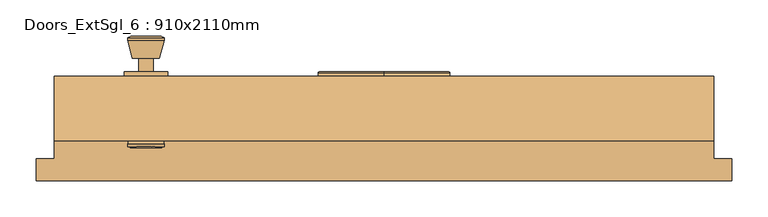
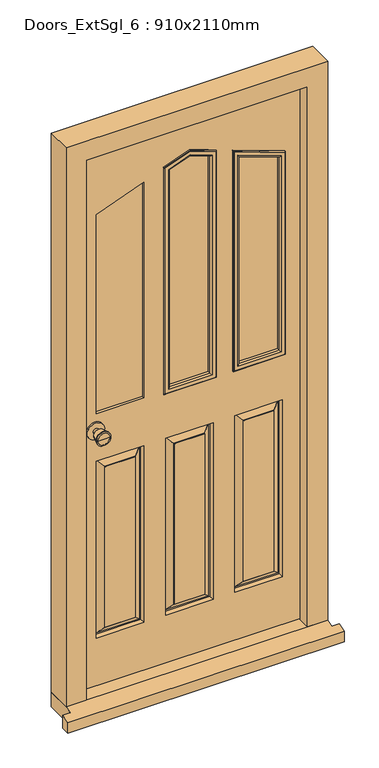
"""IFC4 building model written with IfcOpenShell, lengths in millimetres: door geometry, Doors_ExtSgl_6 : 910x2110mm."""

from ifc_helpers import new_model, si_unit, point, frame, frame_2d, origin, place, context, project, spatial, polyline, circle_curve, ellipse_curve, trimmed, segment, composite_curve, outline, extrude, faceted_brep, source, transform, mapped, element, save
from ifc_brep_helpers import plane_surface, cylinder_surface, revolved_surface, advanced_brep


def doors_extsgl_6_910x2110mm_72be2df1(model_context):
    return source(origin(), model_context, "Body", "SolidModel", [
        advanced_brep(
        [(-328.4666667, 18.4, 1000.0), (-338.4666667, 18.4, 1000.0), (-318.4666667, 18.4, 1000.0), (-307.9907991, 67.4, 1000.0), (-348.9425342, 67.4, 1000.0), (-328.4666667, 67.4, 1000.0), (-303.4666667, 65.5721319, 1000.0), (-353.4666667, 65.5721319, 1000.0), (-303.4666667, 62.1084537, 1000.0), (-353.4666667, 62.1084537, 1000.0), (-309.8304306, 37.4, 1000.0), (-347.1029027, 37.4, 1000.0), (-318.4666667, 37.4, 1000.0), (-338.4666667, 37.4, 1000.0)],
        [
            (0, 1),
            (1, 2, circle_curve(frame((-328.4666667, 18.4, 1000.0), z_axis=(0.0, -1.0, 0.0), x_axis=(-1.0, 0.0, 0.0)), 10.0)),
            (2, 0),
            (2, 1, circle_curve(frame((-328.4666667, 18.4, 1000.0), z_axis=(0.0, -1.0, 0.0), x_axis=(-1.0, 0.0, 0.0)), 10.0)),
            (3, 4, circle_curve(frame((-328.4666667, 67.4, 1000.0), z_axis=(0.0, 1.0, 0.0), x_axis=(-1.0, 0.0, 0.0)), 20.4758676)),
            (4, 5),
            (5, 3),
            (4, 3, circle_curve(frame((-328.4666667, 67.4, 1000.0), z_axis=(0.0, 1.0, 0.0), x_axis=(-1.0, 0.0, 0.0)), 20.4758676)),
            (6, 7, circle_curve(frame((-328.4666667, 65.5721319, 1000.0), z_axis=(0.0, 1.0, 0.0), x_axis=(-1.0, 0.0, 0.0)), 25.0)),
            (7, 4),
            (3, 6),
            (7, 6, circle_curve(frame((-328.4666667, 65.5721319, 1000.0), z_axis=(0.0, 1.0, 0.0), x_axis=(-1.0, 0.0, 0.0)), 25.0)),
            (8, 9, circle_curve(frame((-328.4666667, 62.1084537, 1000.0), z_axis=(0.0, 1.0, 0.0), x_axis=(-1.0, 0.0, 0.0)), 25.0)),
            (9, 7),
            (6, 8),
            (9, 8, circle_curve(frame((-328.4666667, 62.1084537, 1000.0), z_axis=(0.0, 1.0, 0.0), x_axis=(-1.0, 0.0, 0.0)), 25.0)),
            (10, 11, circle_curve(frame((-328.4666667, 37.4, 1000.0), z_axis=(0.0, 1.0, 0.0), x_axis=(-1.0, 0.0, 0.0)), 18.636236)),
            (11, 9),
            (8, 10),
            (11, 10, circle_curve(frame((-328.4666667, 37.4, 1000.0), z_axis=(0.0, 1.0, 0.0), x_axis=(-1.0, 0.0, 0.0)), 18.636236)),
            (12, 13, circle_curve(frame((-328.4666667, 37.4, 1000.0), z_axis=(0.0, 1.0, 0.0), x_axis=(-1.0, 0.0, 0.0)), 10.0)),
            (13, 11),
            (10, 12),
            (13, 12, circle_curve(frame((-328.4666667, 37.4, 1000.0), z_axis=(0.0, 1.0, 0.0), x_axis=(-1.0, 0.0, 0.0)), 10.0)),
            (1, 13),
            (12, 2),
        ],
        [
            plane_surface(frame((-328.4666667, 18.4, 1000.0), z_axis=(0.0, -1.0, 0.0), x_axis=(-1.0, 0.0, 0.0))),
            plane_surface(frame((-328.4666667, 67.4, 1000.0), z_axis=(0.0, 1.0, 0.0), x_axis=(-1.0, 0.0, 0.0))),
            revolved_surface(polyline([(-348.9425342, 67.4, 1000.0), (-353.4666667, 65.5721319, 1000.0)]), (-328.4666667, 18.4, 1000.0), (0.0, -1.0, 0.0)),
            cylinder_surface(frame((-328.4666667, 18.4, 1000.0), z_axis=(0.0, -1.0, 0.0), x_axis=(-1.0, 0.0, 0.0)), 25.0),
            revolved_surface(polyline([(-353.4666667, 62.1084537, 1000.0), (-347.1029027, 37.4, 1000.0)]), (-328.4666667, 18.4, 1000.0), (0.0, -1.0, 0.0)),
            plane_surface(frame((-328.4666667, 37.4, 1000.0), z_axis=(0.0, -1.0, 0.0), x_axis=(-1.0, 0.0, 0.0))),
            cylinder_surface(frame((-328.4666667, 18.4, 1000.0), z_axis=(0.0, -1.0, 0.0), x_axis=(-1.0, 0.0, 0.0)), 10.0),
        ],
        [
            (0, [[1, 2, 3]]),
            (0, [[-3, 4, -1]]),
            (1, [[5, 6, 7]]),
            (1, [[8, -7, -6]]),
            (2, [[9, 10, -5, 11]]),
            (2, [[12, -11, -8, -10]]),
            (3, [[13, 14, -9, 15]]),
            (3, [[16, -15, -12, -14]]),
            (4, [[17, 18, -13, 19]]),
            (4, [[20, -19, -16, -18]]),
            (5, [[21, 22, -17, 23]]),
            (5, [[24, -23, -20, -22]]),
            (6, [[-2, 25, -21, 26]]),
            (6, [[-4, -26, -24, -25]]),
        ],
    ),
        extrude(outline(composite_curve([segment(trimmed(circle_curve(frame_2d((1000.0, -328.4666667)), 30.0), [point((1000.0, -358.4666667))], [point((1000.0, -298.4666667))], False, "CARTESIAN"), True, "CONTINUOUS"), segment(trimmed(circle_curve(frame_2d((1000.0, -328.4666667)), 30.0), [point((1000.0, -298.4666667))], [point((1000.0, -358.4666667))], False, "CARTESIAN"), True, "CONTINUOUS")], self_intersect=False)), frame((0.0, 12.4, 0.0), z_axis=(0.0, 1.0, 0.0), x_axis=(0.0, 0.0, 1.0)), (0.0, 0.0, 1.0), 6.0),
        advanced_brep(
        [(-328.4666667, -37.6, 1000.0), (-318.4666667, -37.6, 1000.0), (-338.4666667, -37.6, 1000.0), (-307.9907991, -86.6, 1000.0), (-328.4666667, -86.6, 1000.0), (-348.9425342, -86.6, 1000.0), (-303.4666667, -84.7721319, 1000.0), (-353.4666667, -84.7721319, 1000.0), (-303.4666667, -81.3084537, 1000.0), (-353.4666667, -81.3084537, 1000.0), (-309.8304306, -56.6, 1000.0), (-347.1029027, -56.6, 1000.0), (-318.4666667, -56.6, 1000.0), (-338.4666667, -56.6, 1000.0)],
        [
            (0, 1),
            (1, 2, circle_curve(frame((-328.4666667, -37.6, 1000.0), z_axis=(0.0, 1.0, 0.0), x_axis=(-1.0, 0.0, 0.0)), 10.0)),
            (2, 0),
            (2, 1, circle_curve(frame((-328.4666667, -37.6, 1000.0), z_axis=(0.0, 1.0, 0.0), x_axis=(-1.0, 0.0, 0.0)), 10.0)),
            (3, 4),
            (4, 5),
            (5, 3, circle_curve(frame((-328.4666667, -86.6, 1000.0), z_axis=(0.0, -1.0, 0.0), x_axis=(-1.0, 0.0, 0.0)), 20.4758676)),
            (3, 5, circle_curve(frame((-328.4666667, -86.6, 1000.0), z_axis=(0.0, -1.0, 0.0), x_axis=(-1.0, 0.0, 0.0)), 20.4758676)),
            (6, 3),
            (5, 7),
            (7, 6, circle_curve(frame((-328.4666667, -84.7721319, 1000.0), z_axis=(0.0, -1.0, 0.0), x_axis=(-1.0, 0.0, 0.0)), 25.0)),
            (6, 7, circle_curve(frame((-328.4666667, -84.7721319, 1000.0), z_axis=(0.0, -1.0, 0.0), x_axis=(-1.0, 0.0, 0.0)), 25.0)),
            (8, 6),
            (7, 9),
            (9, 8, circle_curve(frame((-328.4666667, -81.3084537, 1000.0), z_axis=(0.0, -1.0, 0.0), x_axis=(-1.0, 0.0, 0.0)), 25.0)),
            (8, 9, circle_curve(frame((-328.4666667, -81.3084537, 1000.0), z_axis=(0.0, -1.0, 0.0), x_axis=(-1.0, 0.0, 0.0)), 25.0)),
            (10, 8),
            (9, 11),
            (11, 10, circle_curve(frame((-328.4666667, -56.6, 1000.0), z_axis=(0.0, -1.0, 0.0), x_axis=(-1.0, 0.0, 0.0)), 18.636236)),
            (10, 11, circle_curve(frame((-328.4666667, -56.6, 1000.0), z_axis=(0.0, -1.0, 0.0), x_axis=(-1.0, 0.0, 0.0)), 18.636236)),
            (12, 10),
            (11, 13),
            (13, 12, circle_curve(frame((-328.4666667, -56.6, 1000.0), z_axis=(0.0, -1.0, 0.0), x_axis=(-1.0, 0.0, 0.0)), 10.0)),
            (12, 13, circle_curve(frame((-328.4666667, -56.6, 1000.0), z_axis=(0.0, -1.0, 0.0), x_axis=(-1.0, 0.0, 0.0)), 10.0)),
            (1, 12),
            (13, 2),
        ],
        [
            plane_surface(frame((-328.4666667, -37.6, 1000.0), z_axis=(0.0, 1.0, 0.0), x_axis=(-1.0, 0.0, 0.0))),
            plane_surface(frame((-328.4666667, -86.6, 1000.0), z_axis=(0.0, -1.0, 0.0), x_axis=(-1.0, 0.0, 0.0))),
            revolved_surface(polyline([(-348.9425342, -86.6, 1000.0), (-353.4666667, -84.7721319, 1000.0)]), (-328.4666667, -37.6, 1000.0), (0.0, 1.0, 0.0)),
            cylinder_surface(frame((-328.4666667, -37.6, 1000.0), z_axis=(0.0, 1.0, 0.0), x_axis=(-1.0, 0.0, 0.0)), 25.0),
            revolved_surface(polyline([(-353.4666667, -81.3084537, 1000.0), (-347.1029027, -56.6, 1000.0)]), (-328.4666667, -37.6, 1000.0), (0.0, 1.0, 0.0)),
            plane_surface(frame((-328.4666667, -56.6, 1000.0), z_axis=(0.0, 1.0, 0.0), x_axis=(-1.0, 0.0, 0.0))),
            cylinder_surface(frame((-328.4666667, -37.6, 1000.0), z_axis=(0.0, 1.0, 0.0), x_axis=(-1.0, 0.0, 0.0)), 10.0),
        ],
        [
            (0, [[1, 2, 3]]),
            (0, [[-3, 4, -1]]),
            (1, [[5, 6, 7]]),
            (1, [[-6, -5, 8]]),
            (2, [[9, -7, 10, 11]]),
            (2, [[-10, -8, -9, 12]]),
            (3, [[13, -11, 14, 15]]),
            (3, [[-14, -12, -13, 16]]),
            (4, [[17, -15, 18, 19]]),
            (4, [[-18, -16, -17, 20]]),
            (5, [[21, -19, 22, 23]]),
            (5, [[-22, -20, -21, 24]]),
            (6, [[25, -23, 26, -2]]),
            (6, [[-26, -24, -25, -4]]),
        ],
    ),
        extrude(outline(composite_curve([segment(trimmed(circle_curve(frame_2d((1000.0, -328.4666667)), 30.0), [point((1000.0, -358.4666667))], [point((1000.0, -298.4666667))], False, "CARTESIAN"), True, "CONTINUOUS"), segment(trimmed(circle_curve(frame_2d((1000.0, -328.4666667)), 30.0), [point((1000.0, -298.4666667))], [point((1000.0, -358.4666667))], False, "CARTESIAN"), True, "CONTINUOUS")], self_intersect=False)), frame((0.0, -37.6, 0.0), z_axis=(0.0, 1.0, 0.0), x_axis=(0.0, 0.0, 1.0)), (0.0, 0.0, 1.0), 6.0),
        faceted_brep([(384.5333333, -76.6, 54.5), (384.5333333, -34.6, 54.5), (406.5333333, -34.6, 54.5), (406.5333333, 12.4, 54.5), (455.0333333, 12.4, 54.5), (455.0333333, -76.6, 54.5), (455.0333333, -76.6, 2110.0), (-454.9666667, -76.6, 2110.0), (-454.9666667, -76.6, 54.5), (-384.4666667, -76.6, 54.5), (-384.4666667, -76.6, 2039.5), (384.5333333, -76.6, 2039.5), (455.0333333, 12.4, 2110.0), (406.5333333, 12.4, 2061.5), (-406.4666667, 12.4, 2061.5), (-406.4666667, 12.4, 54.5), (-454.9666667, 12.4, 54.5), (-454.9666667, 12.4, 2110.0), (406.5333333, -34.6, 2061.5), (384.5333333, -34.6, 2039.5), (-384.4666667, -34.6, 2039.5), (-384.4666667, -34.6, 54.5), (-406.4666667, -34.6, 54.5), (-406.4666667, -34.6, 2061.5)], [[[0, 1, 2, 3, 4, 5]], [[5, 6, 7, 8, 9, 10, 11, 0]], [[4, 12, 6, 5]], [[3, 13, 14, 15, 16, 17, 12, 4]], [[2, 18, 13, 3]], [[1, 19, 20, 21, 22, 23, 18, 2]], [[0, 11, 19, 1]], [[9, 21, 20, 10]], [[8, 16, 15, 22, 21, 9]], [[7, 17, 16, 8]], [[14, 23, 22, 15]], [[6, 12, 17, 7]], [[13, 18, 23, 14]], [[10, 20, 19, 11]]]),
        faceted_brep([(403.5333333, 12.4, 58.5), (-404.3916961, 12.4, 58.5), (-404.3916961, 12.4, 2058.5), (403.5333333, 12.4, 2058.5), (-82.8, 12.4, 1058.5), (82.8666667, 12.4, 1058.5), (82.8666667, 12.4, 1878.3511323), (0.0333333, 12.4, 1908.5), (-82.8, 12.4, 1878.3511323), (323.5333333, 12.4, 1058.5), (323.5333333, 12.4, 1790.7556292), (157.8666667, 12.4, 1851.0533647), (157.8666667, 12.4, 1058.5), (-157.8, 12.4, 1851.0533647), (-323.4666667, 12.4, 1790.7556292), (-323.4666667, 12.4, 1058.5), (-157.8, 12.4, 1058.5), (-157.8, 12.4, 883.5), (-323.4666667, 12.4, 883.5), (-323.4666667, 12.4, 233.5), (-157.8, 12.4, 233.5), (323.5333333, 12.4, 883.5), (157.8666667, 12.4, 883.5), (157.8666667, 12.4, 233.5), (323.5333333, 12.4, 233.5), (82.8666667, 12.4, 883.5), (-82.8, 12.4, 883.5), (-82.8, 12.4, 233.5), (82.8666667, 12.4, 233.5), (-187.8, 12.4, 263.5), (-293.4666667, 12.4, 263.5), (-293.4666667, 12.4, 853.5), (-187.8, 12.4, 853.5), (293.5333333, 12.4, 263.5), (187.8666667, 12.4, 263.5), (187.8666667, 12.4, 853.5), (293.5333333, 12.4, 853.5), (52.8666667, 12.4, 263.5), (-52.8, 12.4, 263.5), (-52.8, 12.4, 853.5), (52.8666667, 12.4, 853.5), (403.5333333, -31.6, 58.5), (403.5333333, -31.6, 2058.5), (-404.3916961, -31.6, 2058.5), (-404.3916961, -31.6, 58.5), (-82.8, -31.6, 1058.5), (-82.8, -31.6, 1878.3511323), (0.0333333, -31.6, 1908.5), (82.8666667, -31.6, 1878.3511323), (82.8666667, -31.6, 1058.5), (323.5333333, -31.6, 1058.5), (157.8666667, -31.6, 1058.5), (157.8666667, -31.6, 1851.0533647), (323.5333333, -31.6, 1790.7556292), (-157.8, -31.6, 1851.0533647), (-157.8, -31.6, 1058.5), (-323.4666667, -31.6, 1058.5), (-323.4666667, -31.6, 1790.7556292), (157.8666667, -31.6, 883.5), (323.5333333, -31.6, 883.5), (323.5333333, -31.6, 233.5), (157.8666667, -31.6, 233.5), (-323.4666667, -31.6, 883.5), (-157.8, -31.6, 883.5), (-157.8, -31.6, 233.5), (-323.4666667, -31.6, 233.5), (-82.8, -31.6, 883.5), (82.8666667, -31.6, 883.5), (82.8666667, -31.6, 233.5), (-82.8, -31.6, 233.5), (187.8666667, -31.6, 263.5), (293.5333333, -31.6, 263.5), (293.5333333, -31.6, 853.5), (187.8666667, -31.6, 853.5), (-293.4666667, -31.6, 263.5), (-187.8, -31.6, 263.5), (-187.8, -31.6, 853.5), (-293.4666667, -31.6, 853.5), (-52.8, -31.6, 263.5), (52.8666667, -31.6, 263.5), (52.8666667, -31.6, 853.5), (-52.8, -31.6, 853.5), (160.8666667, -16.6, 880.5), (160.8666667, -16.6, 236.5), (185.8666667, -30.6, 855.5), (165.8666667, -16.6, 875.5), (165.8666667, -16.6, 241.5), (185.8666667, -30.6, 261.5), (187.8666667, -30.6, 853.5), (187.8666667, -30.6, 263.5), (320.5333333, -16.6, 236.5), (315.5333333, -16.6, 241.5), (295.5333333, -30.6, 261.5), (293.5333333, -30.6, 263.5), (320.5333333, -16.6, 880.5), (315.5333333, -16.6, 875.5), (295.5333333, -30.6, 855.5), (293.5333333, -30.6, 853.5), (-320.4666667, -16.6, 880.5), (-320.4666667, -16.6, 236.5), (-295.4666667, -30.6, 855.5), (-315.4666667, -16.6, 875.5), (-315.4666667, -16.6, 241.5), (-295.4666667, -30.6, 261.5), (-293.4666667, -30.6, 853.5), (-293.4666667, -30.6, 263.5), (-160.8, -16.6, 236.5), (-165.8, -16.6, 241.5), (-185.8, -30.6, 261.5), (-187.8, -30.6, 263.5), (-160.8, -16.6, 880.5), (-165.8, -16.6, 875.5), (-185.8, -30.6, 855.5), (-187.8, -30.6, 853.5), (-187.8, 11.4, 263.5), (-187.8, 11.4, 853.5), (-165.8, -2.6, 241.5), (-185.8, 11.4, 261.5), (-185.8, 11.4, 855.5), (-165.8, -2.6, 875.5), (-160.8, -2.6, 236.5), (-160.8, -2.6, 880.5), (-293.4666667, 11.4, 853.5), (-295.4666667, 11.4, 855.5), (-315.4666667, -2.6, 875.5), (-320.4666667, -2.6, 880.5), (-293.4666667, 11.4, 263.5), (-295.4666667, 11.4, 261.5), (-315.4666667, -2.6, 241.5), (-320.4666667, -2.6, 236.5), (320.5333333, -2.6, 880.5), (320.5333333, -2.6, 236.5), (295.5333333, 11.4, 855.5), (315.5333333, -2.6, 875.5), (315.5333333, -2.6, 241.5), (295.5333333, 11.4, 261.5), (293.5333333, 11.4, 853.5), (293.5333333, 11.4, 263.5), (160.8666667, -2.6, 236.5), (165.8666667, -2.6, 241.5), (185.8666667, 11.4, 261.5), (187.8666667, 11.4, 263.5), (160.8666667, -2.6, 880.5), (165.8666667, -2.6, 875.5), (185.8666667, 11.4, 855.5), (187.8666667, 11.4, 853.5), (-52.8, -30.6, 263.5), (-52.8, -30.6, 853.5), (-74.8, -16.6, 241.5), (-54.8, -30.6, 261.5), (-54.8, -30.6, 855.5), (-74.8, -16.6, 875.5), (-79.8, -16.6, 236.5), (-79.8, -16.6, 880.5), (52.8666667, -30.6, 853.5), (54.8666667, -30.6, 855.5), (74.8666667, -16.6, 875.5), (79.8666667, -16.6, 880.5), (52.8666667, -30.6, 263.5), (54.8666667, -30.6, 261.5), (74.8666667, -16.6, 241.5), (79.8666667, -16.6, 236.5), (79.8666667, -2.6, 880.5), (79.8666667, -2.6, 236.5), (54.8666667, 11.4, 855.5), (74.8666667, -2.6, 875.5), (74.8666667, -2.6, 241.5), (54.8666667, 11.4, 261.5), (52.8666667, 11.4, 853.5), (52.8666667, 11.4, 263.5), (-79.8, -2.6, 236.5), (-74.8, -2.6, 241.5), (-54.8, 11.4, 261.5), (-52.8, 11.4, 263.5), (-79.8, -2.6, 880.5), (-74.8, -2.6, 875.5), (-54.8, 11.4, 855.5), (-52.8, 11.4, 853.5)], [[[0, 1, 2, 3], [4, 5, 6, 7, 8], [9, 10, 11, 12], [13, 14, 15, 16], [17, 18, 19, 20], [21, 22, 23, 24], [25, 26, 27, 28]], [[29, 30, 31, 32]], [[33, 34, 35, 36]], [[37, 38, 39, 40]], [[41, 42, 43, 44], [45, 46, 47, 48, 49], [50, 51, 52, 53], [54, 55, 56, 57], [58, 59, 60, 61], [62, 63, 64, 65], [66, 67, 68, 69]], [[70, 71, 72, 73]], [[74, 75, 76, 77]], [[78, 79, 80, 81]], [[3, 42, 41, 0]], [[2, 43, 42, 3]], [[1, 44, 43, 2]], [[0, 41, 44, 1]], [[8, 46, 45, 4]], [[7, 47, 46, 8]], [[6, 48, 47, 7]], [[5, 49, 48, 6]], [[4, 45, 49, 5]], [[12, 51, 50, 9]], [[11, 52, 51, 12]], [[10, 53, 52, 11]], [[9, 50, 53, 10]], [[16, 55, 54, 13]], [[15, 56, 55, 16]], [[14, 57, 56, 15]], [[13, 54, 57, 14]], [[82, 58, 61, 83]], [[84, 85, 86, 87]], [[70, 73, 88, 89]], [[61, 60, 90, 83]], [[86, 91, 92, 87]], [[89, 93, 71, 70]], [[60, 59, 94, 90]], [[91, 95, 96, 92]], [[93, 97, 72, 71]], [[82, 94, 59, 58]], [[83, 90, 94, 82], [85, 95, 91, 86]], [[84, 96, 95, 85]], [[87, 92, 96, 84], [88, 97, 93, 89]], [[73, 72, 97, 88]], [[98, 62, 65, 99]], [[100, 101, 102, 103]], [[74, 77, 104, 105]], [[65, 64, 106, 99]], [[102, 107, 108, 103]], [[105, 109, 75, 74]], [[64, 63, 110, 106]], [[107, 111, 112, 108]], [[109, 113, 76, 75]], [[98, 110, 63, 62]], [[99, 106, 110, 98], [101, 111, 107, 102]], [[100, 112, 111, 101]], [[103, 108, 112, 100], [104, 113, 109, 105]], [[77, 76, 113, 104]], [[114, 29, 32, 115]], [[116, 117, 118, 119]], [[17, 20, 120, 121]], [[32, 31, 122, 115]], [[118, 123, 124, 119]], [[121, 125, 18, 17]], [[31, 30, 126, 122]], [[123, 127, 128, 124]], [[125, 129, 19, 18]], [[114, 126, 30, 29]], [[117, 127, 123, 118], [115, 122, 126, 114]], [[116, 128, 127, 117]], [[120, 129, 125, 121], [119, 124, 128, 116]], [[20, 19, 129, 120]], [[130, 21, 24, 131]], [[132, 133, 134, 135]], [[33, 36, 136, 137]], [[24, 23, 138, 131]], [[134, 139, 140, 135]], [[137, 141, 34, 33]], [[23, 22, 142, 138]], [[139, 143, 144, 140]], [[141, 145, 35, 34]], [[130, 142, 22, 21]], [[131, 138, 142, 130], [133, 143, 139, 134]], [[132, 144, 143, 133]], [[135, 140, 144, 132], [136, 145, 141, 137]], [[36, 35, 145, 136]], [[146, 78, 81, 147]], [[148, 149, 150, 151]], [[66, 69, 152, 153]], [[81, 80, 154, 147]], [[150, 155, 156, 151]], [[153, 157, 67, 66]], [[80, 79, 158, 154]], [[155, 159, 160, 156]], [[157, 161, 68, 67]], [[146, 158, 79, 78]], [[149, 159, 155, 150], [147, 154, 158, 146]], [[148, 160, 159, 149]], [[152, 161, 157, 153], [151, 156, 160, 148]], [[69, 68, 161, 152]], [[162, 25, 28, 163]], [[164, 165, 166, 167]], [[37, 40, 168, 169]], [[28, 27, 170, 163]], [[166, 171, 172, 167]], [[169, 173, 38, 37]], [[27, 26, 174, 170]], [[171, 175, 176, 172]], [[173, 177, 39, 38]], [[162, 174, 26, 25]], [[163, 170, 174, 162], [165, 175, 171, 166]], [[164, 176, 175, 165]], [[167, 172, 176, 164], [168, 177, 173, 169]], [[40, 39, 177, 168]]]),
        faceted_brep([(480.0333333, -131.6, 0.0), (480.0333333, -101.6, 0.0), (480.0333333, -101.6, 47.2703282), (480.0333333, -131.6, 38.5947221), (-479.9666667, -131.6, 38.5947221), (-479.9666667, -101.6, 47.2703282), (-479.9666667, -101.6, 0.0), (-479.9666667, -131.6, 0.0), (-454.9666667, -101.6, 0.0), (-454.9666667, 12.4, 0.0), (455.0333333, 12.4, 0.0), (455.0333333, -101.6, 0.0), (455.0333333, -101.6, 47.2703282), (455.0333333, -76.6, 54.5), (-454.9666667, -76.6, 54.5), (-454.9666667, -101.6, 47.2703282), (455.0333333, 12.4, 54.5), (-454.9666667, 12.4, 54.5)], [[[0, 1, 2, 3]], [[4, 5, 6, 7]], [[7, 6, 8, 9, 10, 11, 1, 0]], [[3, 4, 7, 0]], [[3, 2, 12, 13, 14, 15, 5, 4]], [[14, 13, 16, 17]], [[17, 16, 10, 9]], [[15, 14, 17, 9, 8]], [[8, 6, 5, 15]], [[11, 10, 16, 13, 12]], [[12, 2, 1, 11]]]),
        extrude(outline(polyline([(1058.5, -82.8), (1058.5, 82.8666667), (1878.3511323, 82.8666667), (1908.5, 0.0333333), (1878.3511323, -82.8), (1058.5, -82.8)])), frame((0.0, -21.6, 0.0), z_axis=(0.0, 1.0, 0.0), x_axis=(0.0, 0.0, 1.0)), (0.0, 0.0, 1.0), 24.0),
        extrude(outline(polyline([(1790.7556292, 323.5333333), (1851.0533647, 157.8666667), (1058.5, 157.8666667), (1058.5, 323.5333333), (1790.7556292, 323.5333333)])), frame((0.0, -21.6, 0.0), z_axis=(0.0, 1.0, 0.0), x_axis=(0.0, 0.0, 1.0)), (0.0, 0.0, 1.0), 24.0),
        extrude(outline(polyline([(1058.5, -157.8), (1851.0533647, -157.8), (1790.7556292, -323.4666667), (1058.5, -323.4666667), (1058.5, -157.8)])), frame((0.0, -21.6, 0.0), z_axis=(0.0, 1.0, 0.0), x_axis=(0.0, 0.0, 1.0)), (0.0, 0.0, 1.0), 24.0),
        advanced_brep(
        [(-90.8, -35.6, 1050.5), (-90.8, -35.6, 1883.9527926), (-90.8, -31.6, 1883.9527926), (-90.8, -31.6, 1050.5), (-88.8, -37.6, 1052.5), (-88.8, -37.6, 1882.5523775), (-70.8, -32.6, 1070.5), (-70.8, -32.6, 1869.9486418), (-75.8, -37.6, 1873.4496795), (-75.8, -37.6, 1065.5), (-70.8, -21.6, 1070.5), (-70.8, -21.6, 1869.9486418), (-82.8, -31.6, 1058.5), (-82.8, -31.6, 1878.3511323), (-82.8, -21.6, 1878.3511323), (-82.8, -21.6, 1058.5), (0.0333333, -35.6, 1917.0134222), (0.0333333, -31.6, 1917.0134222), (0.0333333, -37.6, 1914.8850666), (0.0333333, -32.6, 1895.7298667), (0.0333333, -37.6, 1901.0507556), (0.0333333, -21.6, 1895.7298667), (0.0333333, -31.6, 1908.5), (0.0333333, -21.6, 1908.5), (90.8666667, -35.6, 1883.9527926), (90.8666667, -31.6, 1883.9527926), (88.8666667, -37.6, 1882.5523775), (88.8666667, -37.6, 1052.5), (75.8666667, -37.6, 1873.4496795), (75.8666667, -37.6, 1065.5), (70.8666667, -32.6, 1869.9486418), (70.8666667, -21.6, 1869.9486418), (82.8666667, -21.6, 1878.3511323), (82.8666667, -21.6, 1058.5), (70.8666667, -21.6, 1070.5), (82.8666667, -31.6, 1878.3511323), (90.8666667, -31.6, 1050.5), (82.8666667, -31.6, 1058.5), (90.8666667, -35.6, 1050.5), (70.8666667, -32.6, 1070.5)],
        [
            (0, 1),
            (1, 2),
            (2, 3),
            (3, 0),
            (4, 5),
            (5, 1, ellipse_curve(frame((-88.8, -35.6, 1882.5523775), z_axis=(-0.5735764363510456, 0.0, -0.8191520442889918), x_axis=(0.8191520442889916, 0.0, -0.5735764363510464)), 2.4415492, 2.0)),
            (0, 4, ellipse_curve(frame((-88.8, -35.6, 1052.5), z_axis=(-0.7071067811865476, 0.0, 0.7071067811865474), x_axis=(-0.7071067811865472, 0.0, -0.7071067811865478)), 2.8284271, 2.0)),
            (6, 7),
            (7, 8, ellipse_curve(frame((-75.8, -32.6, 1873.4496795), z_axis=(-0.5735764363510456, 0.0, -0.8191520442889918), x_axis=(0.8191520442889916, 0.0, -0.5735764363510464)), 6.1038729, 5.0)),
            (8, 9),
            (9, 6, ellipse_curve(frame((-75.8, -32.6, 1065.5), z_axis=(-0.7071067811865476, 0.0, 0.7071067811865474), x_axis=(-0.7071067811865472, 0.0, -0.7071067811865478)), 7.0710678, 5.0)),
            (10, 11),
            (11, 7),
            (6, 10),
            (12, 13),
            (13, 14),
            (14, 15),
            (15, 12),
            (1, 16),
            (16, 17),
            (17, 2),
            (5, 18),
            (18, 16, ellipse_curve(frame((0.0333333, -35.6, 1914.8850666), z_axis=(-1.0, 0.0, 0.0), x_axis=(0.0, 0.0, -1.0)), 2.1283555, 2.0)),
            (7, 19),
            (19, 20, ellipse_curve(frame((0.0333333, -32.6, 1901.0507556), z_axis=(-1.0, 0.0, 0.0), x_axis=(0.0, 0.0, -1.0)), 5.3208889, 5.0)),
            (20, 8),
            (11, 21),
            (21, 19),
            (13, 22),
            (22, 23),
            (23, 14),
            (16, 24),
            (24, 25),
            (25, 17),
            (18, 26),
            (26, 24, ellipse_curve(frame((88.8666667, -35.6, 1882.5523775), z_axis=(-0.573576436351046, 0.0, 0.8191520442889917), x_axis=(-0.8191520442889921, 0.0, -0.5735764363510458)), 2.4415492, 2.0)),
            (4, 27),
            (27, 26),
            (28, 29),
            (29, 9),
            (20, 28),
            (19, 30),
            (30, 28, ellipse_curve(frame((75.8666667, -32.6, 1873.4496795), z_axis=(-0.573576436351046, 0.0, 0.8191520442889917), x_axis=(-0.8191520442889921, 0.0, -0.5735764363510458)), 6.1038729, 5.0)),
            (21, 31),
            (31, 30),
            (32, 33),
            (33, 15),
            (23, 32),
            (10, 34),
            (34, 31),
            (22, 35),
            (35, 32),
            (25, 36),
            (36, 3),
            (12, 37),
            (37, 35),
            (24, 38),
            (38, 36),
            (27, 38, ellipse_curve(frame((88.8666667, -35.6, 1052.5), z_axis=(0.7071067811865475, 0.0, 0.7071067811865476), x_axis=(-0.7071067811865475, 0.0, 0.7071067811865475)), 2.8284271, 2.0)),
            (30, 39),
            (39, 29, ellipse_curve(frame((75.8666667, -32.6, 1065.5), z_axis=(0.7071067811865475, 0.0, 0.7071067811865476), x_axis=(-0.7071067811865475, 0.0, 0.7071067811865475)), 7.0710678, 5.0)),
            (34, 39),
            (37, 33),
            (38, 0),
            (39, 6),
        ],
        [
            plane_surface(frame((-90.8, -31.6, 1050.5), z_axis=(-1.0, 0.0, 0.0), x_axis=(0.0, 0.0, 1.0))),
            cylinder_surface(frame((-88.8, -35.6, 1058.5), z_axis=(0.0, 0.0, -1.0), x_axis=(-1.0, 0.0, 0.0)), 2.0),
            cylinder_surface(frame((-75.8, -32.6, 1058.5), z_axis=(0.0, 0.0, -1.0), x_axis=(-1.0, 0.0, 0.0)), 5.0),
            plane_surface(frame((-70.8, -32.6, 1070.5), z_axis=(1.0, 0.0, 0.0), x_axis=(0.0, 0.0, 1.0))),
            plane_surface(frame((-82.8, -21.6, 1058.5), z_axis=(-1.0, 0.0, 0.0), x_axis=(0.0, 0.0, 1.0))),
            plane_surface(frame((-90.8, -31.6, 1883.9527926), z_axis=(-0.34202014332566827, 0.0, 0.9396926207859086), x_axis=(0.9396926207859086, 0.0, 0.34202014332566827))),
            cylinder_surface(frame((-84.8521209, -35.6, 1883.989288), z_axis=(-0.9396926207859082, 0.0, -0.34202014332566943), x_axis=(-0.34202014332566943, 0.0, 0.9396926207859082)), 2.0),
            cylinder_surface(frame((-80.405859, -32.6, 1871.7732839), z_axis=(-0.9396926207859082, 0.0, -0.34202014332566943), x_axis=(-0.34202014332566943, 0.0, 0.9396926207859082)), 5.0),
            plane_surface(frame((-70.8, -32.6, 1869.9486418), z_axis=(0.34202014332567066, 0.0, -0.9396926207859078), x_axis=(0.9396926207859078, 0.0, 0.34202014332567066))),
            plane_surface(frame((-82.8, -21.6, 1878.3511323), z_axis=(-0.3420201433256691, 0.0, 0.9396926207859083), x_axis=(0.9396926207859083, 0.0, 0.3420201433256691))),
            plane_surface(frame((0.0333333, -31.6, 1917.0134222), z_axis=(0.342020143325669, 0.0, 0.9396926207859083), x_axis=(0.9396926207859083, 0.0, -0.342020143325669))),
            cylinder_surface(frame((2.0854542, -35.6, 1914.1381557), z_axis=(-0.9396926207859084, 0.0, 0.342020143325669), x_axis=(0.342020143325669, 0.0, 0.9396926207859084)), 2.0),
            plane_surface(frame((0.0333333, -37.6, 1914.8850666), z_axis=(0.0, -1.0000000000000002, 0.0), x_axis=(0.9396926207859082, 0.0, -0.34202014332566943))),
            cylinder_surface(frame((-2.3608077, -32.6, 1901.9221517), z_axis=(-0.9396926207859084, 0.0, 0.342020143325669), x_axis=(0.342020143325669, 0.0, 0.9396926207859084)), 5.0),
            plane_surface(frame((0.0333333, -32.6, 1895.7298667), z_axis=(-0.34202014332566794, 0.0, -0.9396926207859086), x_axis=(0.9396926207859086, 0.0, -0.34202014332566794))),
            plane_surface(frame((0.0333333, -21.6, 1895.7298667), z_axis=(0.0, 1.0000000000000002, 0.0), x_axis=(0.9396926207859088, 0.0, -0.3420201433256679))),
            plane_surface(frame((0.0333333, -21.6, 1908.5), z_axis=(0.342020143325668, 0.0, 0.9396926207859086), x_axis=(0.9396926207859086, 0.0, -0.342020143325668))),
            plane_surface(frame((0.0333333, -31.6, 1908.5), z_axis=(0.0, 1.0, 0.0), x_axis=(0.9396926207859086, 0.0, -0.342020143325668))),
            plane_surface(frame((90.8666667, -31.6, 1883.9527926), z_axis=(1.0, 0.0, 0.0), x_axis=(0.0, 0.0, -1.0))),
            cylinder_surface(frame((88.8666667, -35.6, 1878.3511323), z_axis=(0.0, 0.0, 1.0), x_axis=(1.0, 0.0, 0.0)), 2.0),
            cylinder_surface(frame((75.8666667, -32.6, 1878.3511323), z_axis=(0.0, 0.0, 1.0), x_axis=(1.0, 0.0, 0.0)), 5.0),
            plane_surface(frame((70.8666667, -32.6, 1869.9486418), z_axis=(-1.0, 0.0, 0.0), x_axis=(0.0, 0.0, -1.0))),
            plane_surface(frame((82.8666667, -21.6, 1878.3511323), z_axis=(1.0, 0.0, 0.0), x_axis=(0.0, 0.0, -1.0))),
            plane_surface(frame((90.8666667, -31.6, 1050.5), z_axis=(0.0, 0.0, -1.0), x_axis=(-1.0, 0.0, 0.0))),
            cylinder_surface(frame((82.8666667, -35.6, 1052.5), z_axis=(1.0, 0.0, 0.0), x_axis=(0.0, 0.0, -1.0)), 2.0),
            cylinder_surface(frame((82.8666667, -32.6, 1065.5), z_axis=(1.0, 0.0, 0.0), x_axis=(0.0, 0.0, -1.0)), 5.0),
            plane_surface(frame((70.8666667, -32.6, 1070.5), z_axis=(0.0, 0.0, 1.0), x_axis=(-1.0, 0.0, 0.0))),
            plane_surface(frame((82.8666667, -21.6, 1058.5), z_axis=(0.0, 0.0, -1.0), x_axis=(-1.0, 0.0, 0.0))),
        ],
        [
            (0, [[1, 2, 3, 4]]),
            (1, [[5, 6, -1, 7]]),
            (2, [[8, 9, 10, 11]]),
            (3, [[12, 13, -8, 14]]),
            (4, [[15, 16, 17, 18]]),
            (5, [[19, 20, 21, -2]]),
            (6, [[22, 23, -19, -6]]),
            (7, [[24, 25, 26, -9]]),
            (8, [[27, 28, -24, -13]]),
            (9, [[29, 30, 31, -16]]),
            (10, [[32, 33, 34, -20]]),
            (11, [[35, 36, -32, -23]]),
            (12, [[37, 38, -35, -22, -5], [39, 40, -10, -26, 41]]),
            (13, [[42, 43, -41, -25]]),
            (14, [[44, 45, -42, -28]]),
            (15, [[46, 47, -17, -31, 48], [49, 50, -44, -27, -12]]),
            (16, [[51, 52, -48, -30]]),
            (17, [[53, 54, -3, -21, -34], [55, 56, -51, -29, -15]]),
            (18, [[57, 58, -53, -33]]),
            (19, [[-38, 59, -57, -36]]),
            (20, [[60, 61, -39, -43]]),
            (21, [[-50, 62, -60, -45]]),
            (22, [[-56, 63, -46, -52]]),
            (23, [[64, -4, -54, -58]]),
            (24, [[-37, -7, -64, -59]]),
            (25, [[65, -11, -40, -61]]),
            (26, [[-49, -14, -65, -62]]),
            (27, [[-55, -18, -47, -63]]),
        ],
    ),
        advanced_brep(
        [(90.8666667, 16.4, 1050.5), (90.8666667, 16.4, 1883.9527926), (90.8666667, 12.4, 1883.9527926), (90.8666667, 12.4, 1050.5), (88.8666667, 18.4, 1052.5), (88.8666667, 18.4, 1882.5523775), (70.8666667, 13.4, 1070.5), (70.8666667, 13.4, 1869.9486418), (75.8666667, 18.4, 1873.4496795), (75.8666667, 18.4, 1065.5), (70.8666667, 2.4, 1070.5), (70.8666667, 2.4, 1869.9486418), (82.8666667, 12.4, 1058.5), (82.8666667, 12.4, 1878.3511323), (82.8666667, 2.4, 1878.3511323), (82.8666667, 2.4, 1058.5), (0.0333333, 16.4, 1917.0134222), (0.0333333, 12.4, 1917.0134222), (0.0333333, 18.4, 1914.8850666), (0.0333333, 13.4, 1895.7298667), (0.0333333, 18.4, 1901.0507556), (0.0333333, 2.4, 1895.7298667), (0.0333333, 12.4, 1908.5), (0.0333333, 2.4, 1908.5), (-90.8, 16.4, 1883.9527926), (-90.8, 12.4, 1883.9527926), (-88.8, 18.4, 1882.5523775), (-88.8, 18.4, 1052.5), (-75.8, 18.4, 1873.4496795), (-75.8, 18.4, 1065.5), (-70.8, 13.4, 1869.9486418), (-70.8, 2.4, 1869.9486418), (-82.8, 2.4, 1878.3511323), (-82.8, 2.4, 1058.5), (-70.8, 2.4, 1070.5), (-82.8, 12.4, 1878.3511323), (-90.8, 12.4, 1050.5), (-82.8, 12.4, 1058.5), (-90.8, 16.4, 1050.5), (-70.8, 13.4, 1070.5)],
        [
            (0, 1),
            (1, 2),
            (2, 3),
            (3, 0),
            (4, 5),
            (5, 1, ellipse_curve(frame((88.8666667, 16.4, 1882.5523775), z_axis=(0.5735764363510463, 0.0, -0.8191520442889916), x_axis=(-0.8191520442889915, 0.0, -0.5735764363510464)), 2.4415492, 2.0)),
            (0, 4, ellipse_curve(frame((88.8666667, 16.4, 1052.5), z_axis=(0.7071067811865472, 0.0, 0.7071067811865478), x_axis=(0.7071067811865478, 0.0, -0.7071067811865474)), 2.8284271, 2.0)),
            (6, 7),
            (7, 8, ellipse_curve(frame((75.8666667, 13.4, 1873.4496795), z_axis=(0.5735764363510463, 0.0, -0.8191520442889916), x_axis=(-0.8191520442889915, 0.0, -0.5735764363510464)), 6.1038729, 5.0)),
            (8, 9),
            (9, 6, ellipse_curve(frame((75.8666667, 13.4, 1065.5), z_axis=(0.7071067811865472, 0.0, 0.7071067811865478), x_axis=(0.7071067811865478, 0.0, -0.7071067811865474)), 7.0710678, 5.0)),
            (10, 11),
            (11, 7),
            (6, 10),
            (12, 13),
            (13, 14),
            (14, 15),
            (15, 12),
            (1, 16),
            (16, 17),
            (17, 2),
            (5, 18),
            (18, 16, ellipse_curve(frame((0.0333333, 16.4, 1914.8850666), z_axis=(1.0, 0.0, 0.0), x_axis=(0.0, 0.0, -1.0)), 2.1283555, 2.0)),
            (7, 19),
            (19, 20, ellipse_curve(frame((0.0333333, 13.4, 1901.0507556), z_axis=(1.0, 0.0, 0.0), x_axis=(0.0, 0.0, -1.0)), 5.3208889, 5.0)),
            (20, 8),
            (11, 21),
            (21, 19),
            (13, 22),
            (22, 23),
            (23, 14),
            (16, 24),
            (24, 25),
            (25, 17),
            (18, 26),
            (26, 24, ellipse_curve(frame((-88.8, 16.4, 1882.5523775), z_axis=(0.5735764363510456, 0.0, 0.8191520442889921), x_axis=(0.819152044288992, 0.0, -0.5735764363510455)), 2.4415492, 2.0)),
            (4, 27),
            (27, 26),
            (28, 29),
            (29, 9),
            (20, 28),
            (19, 30),
            (30, 28, ellipse_curve(frame((-75.8, 13.4, 1873.4496795), z_axis=(0.5735764363510456, 0.0, 0.8191520442889921), x_axis=(0.819152044288992, 0.0, -0.5735764363510455)), 6.1038729, 5.0)),
            (21, 31),
            (31, 30),
            (32, 33),
            (33, 15),
            (23, 32),
            (10, 34),
            (34, 31),
            (22, 35),
            (35, 32),
            (25, 36),
            (36, 3),
            (12, 37),
            (37, 35),
            (24, 38),
            (38, 36),
            (27, 38, ellipse_curve(frame((-88.8, 16.4, 1052.5), z_axis=(-0.7071067811865479, 0.0, 0.707106781186547), x_axis=(0.7071067811865468, 0.0, 0.7071067811865481)), 2.8284271, 2.0)),
            (30, 39),
            (39, 29, ellipse_curve(frame((-75.8, 13.4, 1065.5), z_axis=(-0.7071067811865479, 0.0, 0.707106781186547), x_axis=(0.7071067811865468, 0.0, 0.7071067811865481)), 7.0710678, 5.0)),
            (34, 39),
            (37, 33),
            (38, 0),
            (39, 6),
        ],
        [
            plane_surface(frame((90.8666667, 12.4, 1050.5), z_axis=(1.0, 0.0, 0.0), x_axis=(0.0, 0.0, 1.0))),
            cylinder_surface(frame((88.8666667, 16.4, 1058.5), z_axis=(0.0, 0.0, -1.0), x_axis=(1.0, 0.0, 0.0)), 2.0),
            cylinder_surface(frame((75.8666667, 13.4, 1058.5), z_axis=(0.0, 0.0, -1.0), x_axis=(1.0, 0.0, 0.0)), 5.0),
            plane_surface(frame((70.8666667, 13.4, 1070.5), z_axis=(-1.0, 0.0, 0.0), x_axis=(0.0, 0.0, 1.0))),
            plane_surface(frame((82.8666667, 2.4, 1058.5), z_axis=(1.0, 0.0, 0.0), x_axis=(0.0, 0.0, 1.0))),
            plane_surface(frame((90.8666667, 12.4, 1883.9527926), z_axis=(0.3420201433256677, 0.0, 0.9396926207859089), x_axis=(-0.9396926207859089, 0.0, 0.3420201433256677))),
            cylinder_surface(frame((84.9187875, 16.4, 1883.989288), z_axis=(0.9396926207859085, 0.0, -0.34202014332566855), x_axis=(0.34202014332566855, 0.0, 0.9396926207859085)), 2.0),
            cylinder_surface(frame((80.4725257, 13.4, 1871.7732839), z_axis=(0.9396926207859085, 0.0, -0.34202014332566855), x_axis=(0.34202014332566855, 0.0, 0.9396926207859085)), 5.0),
            plane_surface(frame((70.8666667, 13.4, 1869.9486418), z_axis=(-0.3420201433256698, 0.0, -0.939692620785908), x_axis=(-0.939692620785908, 0.0, 0.3420201433256698))),
            plane_surface(frame((82.8666667, 2.4, 1878.3511323), z_axis=(0.34202014332566855, 0.0, 0.9396926207859085), x_axis=(-0.9396926207859085, 0.0, 0.34202014332566855))),
            plane_surface(frame((0.0333333, 12.4, 1917.0134222), z_axis=(-0.3420201433256698, 0.0, 0.9396926207859081), x_axis=(-0.9396926207859081, 0.0, -0.3420201433256698))),
            cylinder_surface(frame((-2.0187875, 16.4, 1914.1381557), z_axis=(0.9396926207859082, 0.0, 0.3420201433256693), x_axis=(-0.3420201433256693, 0.0, 0.9396926207859082)), 2.0),
            plane_surface(frame((0.0333333, 18.4, 1914.8850666), z_axis=(0.0, 1.0, 0.0), x_axis=(-0.939692620785908, 0.0, -0.34202014332566993))),
            cylinder_surface(frame((2.4274743, 13.4, 1901.9221517), z_axis=(0.9396926207859082, 0.0, 0.3420201433256693), x_axis=(-0.3420201433256693, 0.0, 0.9396926207859082)), 5.0),
            plane_surface(frame((0.0333333, 13.4, 1895.7298667), z_axis=(0.34202014332566916, 0.0, -0.9396926207859082), x_axis=(-0.9396926207859082, 0.0, -0.34202014332566916))),
            plane_surface(frame((0.0333333, 2.4, 1895.7298667), z_axis=(0.0, -1.0, 0.0), x_axis=(-0.9396926207859082, 0.0, -0.3420201433256692))),
            plane_surface(frame((0.0333333, 2.4, 1908.5), z_axis=(-0.3420201433256711, 0.0, 0.9396926207859075), x_axis=(-0.9396926207859075, 0.0, -0.3420201433256711))),
            plane_surface(frame((0.0333333, 12.4, 1908.5), z_axis=(0.0, -1.0, 0.0), x_axis=(-0.9396926207859075, 0.0, -0.3420201433256711))),
            plane_surface(frame((-90.8, 12.4, 1883.9527926), z_axis=(-1.0, 0.0, 0.0), x_axis=(0.0, 0.0, -1.0))),
            cylinder_surface(frame((-88.8, 16.4, 1878.3511323), z_axis=(0.0, 0.0, 1.0), x_axis=(-1.0, 0.0, 0.0)), 2.0),
            cylinder_surface(frame((-75.8, 13.4, 1878.3511323), z_axis=(0.0, 0.0, 1.0), x_axis=(-1.0, 0.0, 0.0)), 5.0),
            plane_surface(frame((-70.8, 13.4, 1869.9486418), z_axis=(1.0, 0.0, 0.0), x_axis=(0.0, 0.0, -1.0))),
            plane_surface(frame((-82.8, 2.4, 1878.3511323), z_axis=(-1.0, 0.0, 0.0), x_axis=(0.0, 0.0, -1.0))),
            plane_surface(frame((-90.8, 12.4, 1050.5), z_axis=(0.0, 0.0, -1.0), x_axis=(1.0, 0.0, 0.0))),
            cylinder_surface(frame((-82.8, 16.4, 1052.5), z_axis=(-1.0, 0.0, 0.0), x_axis=(0.0, 0.0, -1.0)), 2.0),
            cylinder_surface(frame((-82.8, 13.4, 1065.5), z_axis=(-1.0, 0.0, 0.0), x_axis=(0.0, 0.0, -1.0)), 5.0),
            plane_surface(frame((-70.8, 13.4, 1070.5), z_axis=(0.0, 0.0, 1.0), x_axis=(1.0, 0.0, 0.0))),
            plane_surface(frame((-82.8, 2.4, 1058.5), z_axis=(0.0, 0.0, -1.0), x_axis=(1.0, 0.0, 0.0))),
        ],
        [
            (0, [[1, 2, 3, 4]]),
            (1, [[5, 6, -1, 7]]),
            (2, [[8, 9, 10, 11]]),
            (3, [[12, 13, -8, 14]]),
            (4, [[15, 16, 17, 18]]),
            (5, [[19, 20, 21, -2]]),
            (6, [[22, 23, -19, -6]]),
            (7, [[24, 25, 26, -9]]),
            (8, [[27, 28, -24, -13]]),
            (9, [[29, 30, 31, -16]]),
            (10, [[32, 33, 34, -20]]),
            (11, [[35, 36, -32, -23]]),
            (12, [[37, 38, -35, -22, -5], [39, 40, -10, -26, 41]]),
            (13, [[42, 43, -41, -25]]),
            (14, [[44, 45, -42, -28]]),
            (15, [[46, 47, -17, -31, 48], [49, 50, -44, -27, -12]]),
            (16, [[51, 52, -48, -30]]),
            (17, [[53, 54, -3, -21, -34], [55, 56, -51, -29, -15]]),
            (18, [[57, 58, -53, -33]]),
            (19, [[-38, 59, -57, -36]]),
            (20, [[60, 61, -39, -43]]),
            (21, [[-50, 62, -60, -45]]),
            (22, [[-56, 63, -46, -52]]),
            (23, [[64, -4, -54, -58]]),
            (24, [[-37, -7, -64, -59]]),
            (25, [[65, -11, -40, -61]]),
            (26, [[-49, -14, -65, -62]]),
            (27, [[-55, -18, -47, -63]]),
        ],
    ),
        advanced_brep(
        [(331.5333333, -35.6, 1796.3572895), (331.5333333, -35.6, 1050.5), (331.5333333, -31.6, 1050.5), (331.5333333, -31.6, 1796.3572895), (329.5333333, -37.6, 1794.9568744), (329.5333333, -37.6, 1052.5), (311.5333333, -32.6, 1782.3531388), (311.5333333, -32.6, 1070.5), (316.5333333, -37.6, 1065.5), (316.5333333, -37.6, 1785.8541764), (311.5333333, -21.6, 1782.3531388), (311.5333333, -21.6, 1070.5), (323.5333333, -31.6, 1790.7556292), (323.5333333, -31.6, 1058.5), (323.5333333, -21.6, 1058.5), (323.5333333, -21.6, 1790.7556292), (149.8666667, -35.6, 1050.5), (149.8666667, -31.6, 1050.5), (151.8666667, -37.6, 1052.5), (169.8666667, -32.6, 1070.5), (164.8666667, -37.6, 1065.5), (169.8666667, -21.6, 1070.5), (157.8666667, -31.6, 1058.5), (157.8666667, -21.6, 1058.5), (149.8666667, -35.6, 1862.4785487), (149.8666667, -31.6, 1862.4785487), (151.8666667, -37.6, 1859.6222527), (169.8666667, -32.6, 1833.9155886), (164.8666667, -37.6, 1841.0563286), (169.8666667, -21.6, 1833.9155886), (157.8666667, -31.6, 1851.0533647), (157.8666667, -21.6, 1851.0533647)],
        [
            (0, 1),
            (1, 2),
            (2, 3),
            (3, 0),
            (4, 5),
            (5, 1, ellipse_curve(frame((329.5333333, -35.6, 1052.5), z_axis=(0.7071067811865475, 0.0, 0.7071067811865475), x_axis=(-0.7071067811865474, 0.0, 0.7071067811865476)), 2.8284271, 2.0)),
            (0, 4, ellipse_curve(frame((329.5333333, -35.6, 1794.9568744), z_axis=(0.5735764363510453, 0.0, -0.8191520442889922), x_axis=(0.8191520442889922, 0.0, 0.5735764363510456)), 2.4415492, 2.0)),
            (6, 7),
            (7, 8, ellipse_curve(frame((316.5333333, -32.6, 1065.5), z_axis=(0.7071067811865475, 0.0, 0.7071067811865475), x_axis=(-0.7071067811865474, 0.0, 0.7071067811865476)), 7.0710678, 5.0)),
            (8, 9),
            (9, 6, ellipse_curve(frame((316.5333333, -32.6, 1785.8541764), z_axis=(0.5735764363510453, 0.0, -0.8191520442889922), x_axis=(0.8191520442889922, 0.0, 0.5735764363510456)), 6.1038729, 5.0)),
            (10, 11),
            (11, 7),
            (6, 10),
            (12, 13),
            (13, 14),
            (14, 15),
            (15, 12),
            (1, 16),
            (16, 17),
            (17, 2),
            (5, 18),
            (18, 16, ellipse_curve(frame((151.8666667, -35.6, 1052.5), z_axis=(0.7071067811865475, 0.0, -0.7071067811865475), x_axis=(0.7071067811865476, 0.0, 0.7071067811865474)), 2.8284271, 2.0)),
            (7, 19),
            (19, 20, ellipse_curve(frame((164.8666667, -32.6, 1065.5), z_axis=(0.7071067811865475, 0.0, -0.7071067811865475), x_axis=(0.7071067811865476, 0.0, 0.7071067811865474)), 7.0710678, 5.0)),
            (20, 8),
            (11, 21),
            (21, 19),
            (13, 22),
            (22, 23),
            (23, 14),
            (16, 24),
            (24, 25),
            (25, 17),
            (18, 26),
            (26, 24, ellipse_curve(frame((151.8666667, -35.6, 1859.6222527), z_axis=(-0.8191520442889922, 0.0, -0.5735764363510453), x_axis=(0.5735764363510452, 0.0, -0.8191520442889924)), 3.4868936, 2.0)),
            (19, 27),
            (27, 28, ellipse_curve(frame((164.8666667, -32.6, 1841.0563286), z_axis=(-0.8191520442889922, 0.0, -0.5735764363510453), x_axis=(0.5735764363510452, 0.0, -0.8191520442889924)), 8.717234, 5.0)),
            (28, 20),
            (21, 29),
            (29, 27),
            (22, 30),
            (30, 31),
            (31, 23),
            (24, 0),
            (3, 25),
            (26, 4),
            (28, 9),
            (27, 6),
            (29, 10),
            (31, 15),
            (30, 12),
        ],
        [
            plane_surface(frame((331.5333333, -31.6, 1796.3572895), z_axis=(1.0, 0.0, 0.0), x_axis=(0.0, 0.0, -1.0))),
            cylinder_surface(frame((329.5333333, -35.6, 1790.7556292), z_axis=(0.0, 0.0, 1.0), x_axis=(1.0, 0.0, 0.0)), 2.0),
            cylinder_surface(frame((316.5333333, -32.6, 1790.7556292), z_axis=(0.0, 0.0, 1.0), x_axis=(1.0, 0.0, 0.0)), 5.0),
            plane_surface(frame((311.5333333, -32.6, 1782.3531388), z_axis=(-1.0, 0.0, 0.0), x_axis=(0.0, 0.0, -1.0))),
            plane_surface(frame((323.5333333, -21.6, 1790.7556292), z_axis=(1.0, 0.0, 0.0), x_axis=(0.0, 0.0, -1.0))),
            plane_surface(frame((331.5333333, -31.6, 1050.5), z_axis=(0.0, 0.0, -1.0), x_axis=(-1.0, 0.0, 0.0))),
            cylinder_surface(frame((323.5333333, -35.6, 1052.5), z_axis=(1.0, 0.0, 0.0), x_axis=(0.0, 0.0, -1.0)), 2.0),
            cylinder_surface(frame((323.5333333, -32.6, 1065.5), z_axis=(1.0, 0.0, 0.0), x_axis=(0.0, 0.0, -1.0)), 5.0),
            plane_surface(frame((311.5333333, -32.6, 1070.5), z_axis=(0.0, 0.0, 1.0), x_axis=(-1.0, 0.0, 0.0))),
            plane_surface(frame((323.5333333, -21.6, 1058.5), z_axis=(0.0, 0.0, -1.0), x_axis=(-1.0, 0.0, 0.0))),
            plane_surface(frame((149.8666667, -31.6, 1050.5), z_axis=(-1.0, 0.0, 0.0), x_axis=(0.0, 0.0, 1.0))),
            cylinder_surface(frame((151.8666667, -35.6, 1058.5), z_axis=(0.0, 0.0, -1.0), x_axis=(-1.0, 0.0, 0.0)), 2.0),
            cylinder_surface(frame((164.8666667, -32.6, 1058.5), z_axis=(0.0, 0.0, -1.0), x_axis=(-1.0, 0.0, 0.0)), 5.0),
            plane_surface(frame((169.8666667, -32.6, 1070.5), z_axis=(1.0, 0.0, 0.0), x_axis=(0.0, 0.0, 1.0))),
            plane_surface(frame((157.8666667, -21.6, 1058.5), z_axis=(-1.0, 0.0, 0.0), x_axis=(0.0, 0.0, 1.0))),
            plane_surface(frame((149.8666667, -31.6, 1862.4785487), z_axis=(0.3420201433256702, 0.0, 0.9396926207859079), x_axis=(0.9396926207859079, 0.0, -0.3420201433256702))),
            cylinder_surface(frame((159.9187875, -35.6, 1856.6915204), z_axis=(-0.9396926207859078, 0.0, 0.34202014332567043), x_axis=(0.34202014332567043, 0.0, 0.9396926207859078)), 2.0),
            plane_surface(frame((151.8666667, -37.6, 1859.6222527), z_axis=(0.0, -1.0, 0.0), x_axis=(0.9396926207859079, 0.0, -0.34202014332567016))),
            cylinder_surface(frame((155.4725257, -32.6, 1844.4755163), z_axis=(-0.9396926207859078, 0.0, 0.34202014332567043), x_axis=(0.34202014332567043, 0.0, 0.9396926207859078)), 5.0),
            plane_surface(frame((169.8666667, -32.6, 1833.9155886), z_axis=(-0.34202014332566977, 0.0, -0.939692620785908), x_axis=(0.939692620785908, 0.0, -0.34202014332566977))),
            plane_surface(frame((169.8666667, -21.6, 1833.9155886), z_axis=(0.0, 1.0, 0.0), x_axis=(0.9396926207859078, 0.0, -0.3420201433256705))),
            plane_surface(frame((157.8666667, -21.6, 1851.0533647), z_axis=(0.3420201433256704, 0.0, 0.9396926207859079), x_axis=(0.9396926207859079, 0.0, -0.3420201433256704))),
            plane_surface(frame((157.8666667, -31.6, 1851.0533647), z_axis=(0.0, 1.0000000000000002, 0.0), x_axis=(0.9396926207859079, 0.0, -0.3420201433256703))),
        ],
        [
            (0, [[1, 2, 3, 4]]),
            (1, [[5, 6, -1, 7]]),
            (2, [[8, 9, 10, 11]]),
            (3, [[12, 13, -8, 14]]),
            (4, [[15, 16, 17, 18]]),
            (5, [[19, 20, 21, -2]]),
            (6, [[22, 23, -19, -6]]),
            (7, [[24, 25, 26, -9]]),
            (8, [[27, 28, -24, -13]]),
            (9, [[29, 30, 31, -16]]),
            (10, [[32, 33, 34, -20]]),
            (11, [[35, 36, -32, -23]]),
            (12, [[37, 38, 39, -25]]),
            (13, [[40, 41, -37, -28]]),
            (14, [[42, 43, 44, -30]]),
            (15, [[45, -4, 46, -33]]),
            (16, [[47, -7, -45, -36]]),
            (17, [[-5, -47, -35, -22], [-10, -26, -39, 48]]),
            (18, [[49, -11, -48, -38]]),
            (19, [[50, -14, -49, -41]]),
            (20, [[-17, -31, -44, 51], [-12, -50, -40, -27]]),
            (21, [[52, -18, -51, -43]]),
            (22, [[-3, -21, -34, -46], [-15, -52, -42, -29]]),
        ],
    ),
    ])


if __name__ == "__main__":
    model = new_model("IFC4")
    model_context = context("Model", 3, world=origin())
    ifc_project = project(units=[si_unit("LENGTHUNIT", "METRE", prefix="MILLI")], contexts=[model_context])
    site = spatial("IfcSite", under=ifc_project)
    building = spatial("IfcBuilding", under=site)
    placement = place(None, origin())
    doors_extsgl_6_910x2110mm_shape = doors_extsgl_6_910x2110mm_72be2df1(model_context)
    element("IfcDoor", 1, ObjectType="Doors_ExtSgl_6 : 910x2110mm", at=placement, inside=building, context=model_context, shape_type="MappedRepresentation", body=[
        mapped(doors_extsgl_6_910x2110mm_shape, transform((0.0, 0.0, 0.0), x_axis=(1.0, 0.0, 0.0), y_axis=(0.0, 1.0, 0.0), z_axis=(0.0, 0.0, 1.0))),
    ])
    save(model, "model.ifc")

# Revit data of these elements
# Type "Doors_ExtSgl_6 : 910x2110mm"
#   Type Mark = "13"
#   Type Comments = "External Single"
#   Operation = "SingleSwingRight"
#   Construction Type Id = "SGL"
#   Keynote = "L20"
#   Analytic Construction = "Large single-glazed windows"
#   Wrap Layers (Int) from Ext = 0' - 6.98819"
#   Wrap Layers (Ext) from Ext = 0' - 4.03543"
#   Visual Light Transmittance = 0.9
#   Thickness = 0' - 1.73228"
#   Stile Top of Lock rail = 3' - 3.37008"
#   Stile Top Rail = 0' - 5.90551"
#   Stile Shutting = 0' - 3.14961"
#   Stile Muntin Rail = 0' - 2.95276"
#   Stile Lock Rail = 0' - 6.88976"
#   Stile Hanging = 0' - 3.14961"
#   Stile Bottom Rail = 0' - 6.88976"
#   Solar Heat Gain Coefficient = 0.86
#   Rough Width = 2' - 11.82677"
#   Rough Height = 6' - 11.07087"
#   O/A Frame Width = 0' - 2.51969"
#   Heat Transfer Coefficient (U) = 0.979472 BTU/(h·ft²·°F)
#   Handle Z Distance = 3' - 3.37008"
#   Glazing Thickness = 0' - 0.94488"
#   FrameWidth = 0' - 1.65354"
#   FrameOffset - External = 0' - 0.98425"
#   FrameDepth = 0' - 3.50394"
#   Door Panel Width = 2' - 7.77165"
#   Door Panel Thickness = 0' - 1.73228"
#   Door Panel Height = 6' - 6.74016"
#   DONT CHANGE - Panel Width = 0' - 6.52231"
#   Cill Thickness = 0' - 2.14567"
#   Cill Projection = 0' - 1.1811"
#   Handle X Distance = 0' - 2.95276"
#   Height = 6' - 11.07087"
#   Structural Tolerance = 0' - 0.25591"
#   Tolerance = 0' - 0.11811"
#   Undercut = 0' - 0.15748"
#   Width = 2' - 11.82677"
#   Cill Extension = 0' - 0.98425"
#   Cavity Closer Width = 0' - 1.9685"
#   Cavity Closer Offset from Ext = 0' - 4.03543"
#   Cavity Closer Depth = 0' - 3.34646"
#   Vis - Ironmongery = yes
#   Vis - Cavity Closers = yes
#   Define Thermal Properties by = 1
#   Function = 1
#   Material Glass = Door - Glazing
#   Material Door = Door - Panel
#   Material Frame = Door - Frame/Mullion
#   Material Ironmongery = Door - Handle
#   Wall Closure = (empty or 0)
# Element 1 (IfcDoor, "Doors_ExtSgl_6 : 910x2110mm")
#   Materials on its faces: "Door - Panel", "Door - Handle", "Door - Frame/Mullion", "Door - Glazing"
# Materials
#   "Door - Glazing": colour RGB 0 0 255, transparency 0.75
#   "Door - Panel": class "Wood", colour RGB 210 159 95, transparency 0, Cost = 0
#   "Door - Frame/Mullion": class "Wood", colour RGB 212 179 113, transparency 0
#   "Door - Handle": colour RGB 0 0 0, transparency 0
